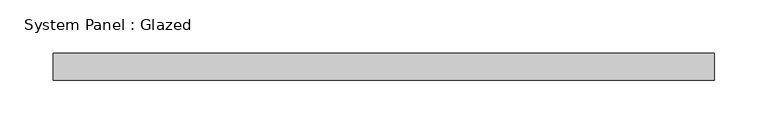
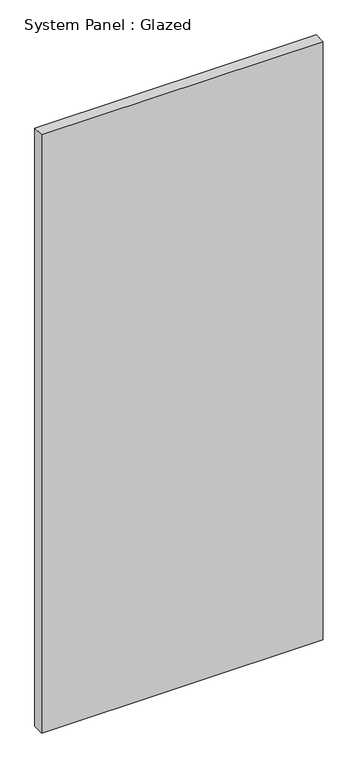
"""IFC4 building model written with IfcOpenShell, lengths in millimetres: plate geometry, System Panel : Glazed."""

from ifc_helpers import new_model, si_unit, origin, origin_with_axes, place, context, project, spatial, polyline, outline, extrude, source, transform, mapped, element, save


def system_panel_glazed_5827f34b(model_context):
    return source(origin(), model_context, "Body", "SweptSolid", [
        extrude(outline(polyline([(311.15, 19.05), (-311.15, 19.05), (-311.15, 44.45), (311.15, 44.45), (311.15, 19.05)])), origin_with_axes(), (0.0, 0.0, 1.0), 1397.0),
    ])


if __name__ == "__main__":
    model = new_model("IFC4")
    model_context = context("Model", 3, world=origin())
    ifc_project = project(units=[si_unit("LENGTHUNIT", "METRE", prefix="MILLI")], contexts=[model_context])
    site = spatial("IfcSite", under=ifc_project)
    building = spatial("IfcBuilding", under=site)
    placement = place(None, origin())
    system_panel_glazed_shape = system_panel_glazed_5827f34b(model_context)
    element("IfcPlate", 1, ObjectType="System Panel : Glazed", at=placement, inside=building, context=model_context, shape_type="MappedRepresentation", body=[
        mapped(system_panel_glazed_shape, transform((0.0, 0.0, 0.0), x_axis=(1.0, 0.0, 0.0), y_axis=(0.0, 1.0, 0.0), z_axis=(0.0, 0.0, 1.0))),
    ])
    save(model, "model.ifc")

# Revit data of these elements
# Type "System Panel : Glazed"
#   Construction Type Id = "GSP4R"
#   Analytic Construction = "1/8 in Pilkington single glazing"
#   Visual Light Transmittance = 0.9
#   Solar Heat Gain Coefficient = 0.86
#   Heat Transfer Coefficient (U) = 1.18115 BTU/(h·ft²·°F)
#   Define Thermal Properties by = 1
# Element 1 (IfcPlate, "System Panel : Glazed")
#   Materials on its faces: "Glass"
# Materials
#   "Glass": class "Glass", colour RGB 0 128 192, transparency 0.75, Description = "Soda Lime Glass", Cost = 0
